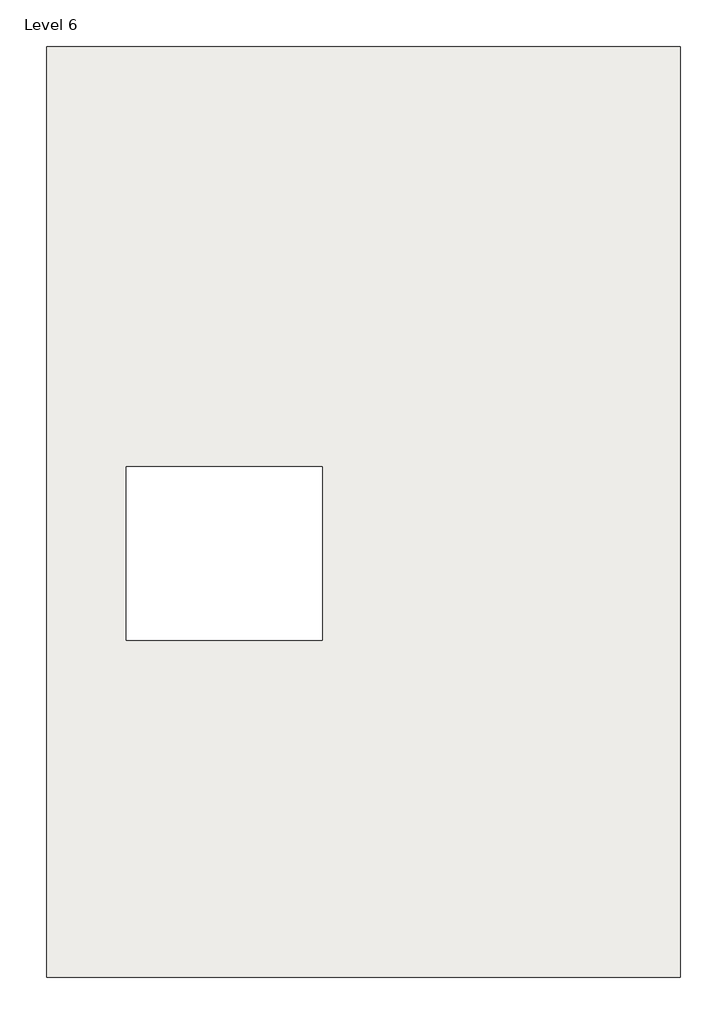
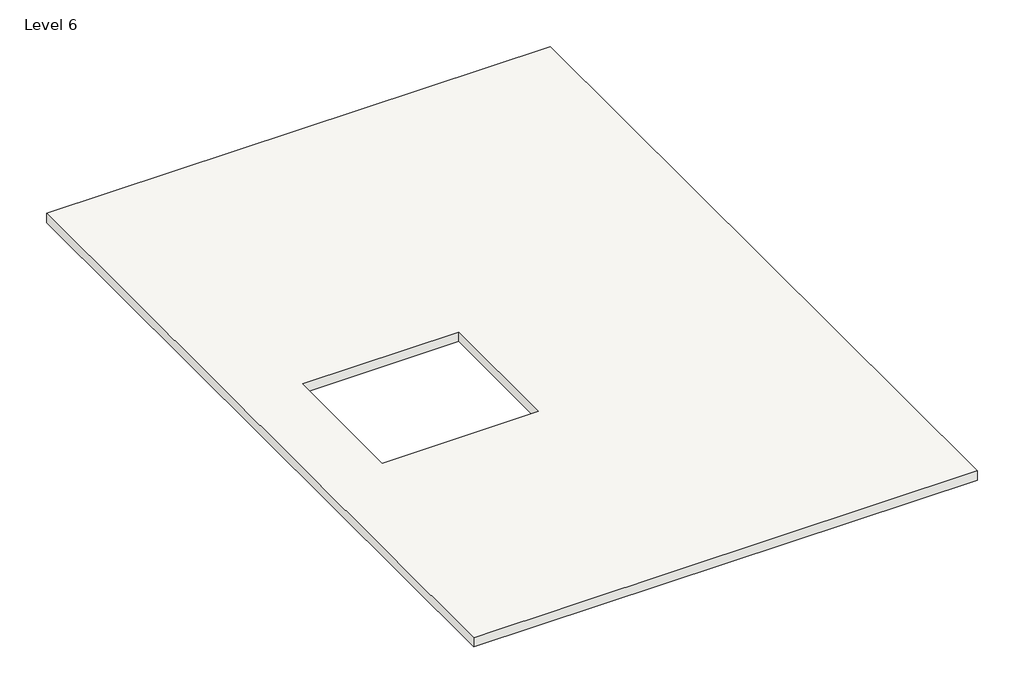
# One storey, incomplete: 1 roof.
"""IFC4 building model written with IfcOpenShell, lengths in millimetres."""

from ifc_helpers import new_model, si_unit, frame, origin, place, context, project, spatial, polyline, outline, extrude, element, save

model = new_model("IFC4")

# Units and contexts
model_context = context("Model", 3, world=origin())
ifc_project = project(units=[si_unit("LENGTHUNIT", "METRE", prefix="MILLI")], contexts=[model_context])

# Site, building, storey
site = spatial("IfcSite", under=ifc_project)
building = spatial("IfcBuilding", under=site)
storey = spatial("IfcBuildingStorey", under=building, Name="Level 6", Elevation=12801.6)

# Roof
placement = place(None, origin())
element("IfcRoof", 1, ObjectType="Generic - 12\"", at=placement, inside=storey, context=model_context, shape_type="SweptSolid", body=[
    extrude(outline(polyline([(2670.5550833, -5508.2570853), (-5216.1449167, -5508.2570853), (-5216.1449167, 6076.3773594), (2670.5550833, 6076.3773594), (2670.5550833, -5508.2570853)]), holes=[polyline([(-1783.4132248, 848.0929147), (-4225.5449167, 848.0929147), (-4225.5449167, -1310.9070853), (-1783.4132248, -1310.9070853), (-1783.4132248, 848.0929147)])]), frame((0.0, 0.0, 12649.2), z_axis=(0.0, 0.0, 1.0), x_axis=(1.0, 0.0, 0.0)), (0.0, 0.0, 1.0), 152.4),
])

save(model, "model.ifc")

# Revit data of these elements
# Type "Generic - 12\""
#   Assembly Code = "B1020"
#   Layers, outside or top first: 0' - 6" no material (function 1)
# Element 1 (IfcRoof, "Generic - 12\"")
#   built-in parameter 1001705 = 42 (stored number, unit not read)
#   built-in parameter 1001701 = -0.5 (stored number, unit not read)
#   built-in parameter 1001710 = 33615
#   Phase Created = New Construction
#   Materials on its faces: "Default Roof"
# Materials
#   "Default Roof": colour RGB 88 101 114, transparency 0, Cost = 0
